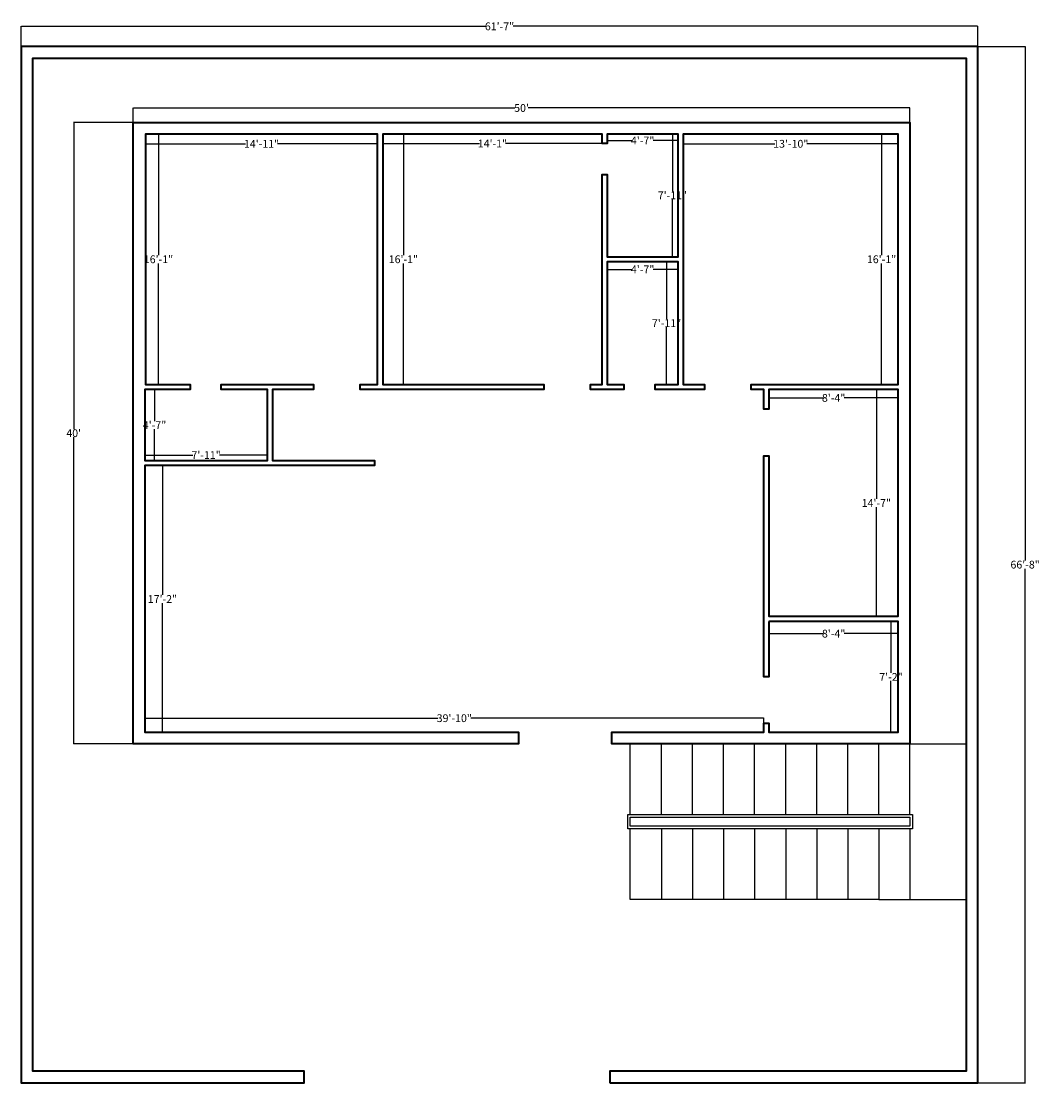
# Model space of a CAD drawing. Units: feet. Extents: x 3511 to 6270, y 2172 to 4127.
# Tile 1 of 4: x 3511 to 4297, y 3307 to 4127. Entities that reach past the tile are written whole.
import ezdxf

# ---------------------------------------------------------------- set-up
doc = ezdxf.new("R2010")
doc.units = ezdxf.units.FT
for name, color, linetype, lineweight in [('A-ANNO-DIMS', 2, 'Continuous', 18), ('A-FLOR-STRS', 4, 'Continuous', 25), ('A-WALL', 7, 'Continuous', 35), ('C-PROP', 1, 'Continuous', 35)]:
    doc.layers.add(name, color=color, linetype=linetype, lineweight=lineweight)
doc.styles.get("Standard").update_dxf_attribs({"font": 'arial.ttf'})
doc.dimstyles.get("Standard").update_dxf_attribs({"dimtxt": 6, "dimasz": 0.18, "dimexe": 0.18, "dimexo": 0.0625, "dimgap": 0.09, "dimtad": 0, "dimtih": 1, "dimtoh": 1, "dimdec": 0, "dimzin": 0, "dimdsep": 46, "dimlunit": 3, "dimtxsty": 'Standard', "dimcen": 0.09, "dimadec": 0, "dimazin": 0, "dimtfac": 1, "dimtdec": 0, "dimtofl": 0, "dimtmove": 0, "dimatfit": 3, "dimfxl": 1, "dimtolj": 1, "dimtzin": 0, "dimarcsym": 0})

# ---------------------------------------------------------------- blocks, each defined once
blk = doc.blocks.new('*D1')
at = {"layer": 'A-ANNO-DIMS', "color": 0, "lineweight": -2, "transparency": 16777216}
for p, q in [((3510.75, 4107.25), (3510.75, 4122.96)), ((3510.93, 4122.78), (3869.76, 4122.78)), ((4249.42, 4122.78), (3890.59, 4122.78)), ((4249.6, 4107.25), (4249.6, 4122.96))]:
    blk.add_line(p, q, dxfattribs=at)
at = {"layer": 'A-ANNO-DIMS', "color": 0, "transparency": 16777216}
for points in [[(3510.93, 4122.81), (3510.93, 4122.75), (3510.75, 4122.78)], [(4249.42, 4122.81), (4249.42, 4122.75), (4249.6, 4122.78)]]:
    blk.add_solid(points, dxfattribs=at)
at = {"layer": 'Defpoints', "color": 0, "transparency": 16777216}
for p in [(4249.6, 4122.78), (3510.75, 4107.19), (4249.6, 4107.19)]:
    blk.add_point(p, dxfattribs=at)
at = {"layer": 'A-ANNO-DIMS', "color": 0, "transparency": 16777216, "insert": (3880.17, 4122.78), "char_height": 6, "attachment_point": 5}
blk.add_mtext('\\A1;61\'-7"', dxfattribs=at)
blk = doc.blocks.new('*D2')
at = {"layer": 'A-ANNO-DIMS', "color": 0, "lineweight": -2, "transparency": 16777216}
for p, q in [((4249.67, 4107.19), (4286.32, 4107.19)), ((4286.14, 4107.01), (4286.14, 3710.22)), ((4286.14, 3307.12), (4286.14, 3703.91)), ((4249.67, 3306.94), (4286.32, 3306.94))]:
    blk.add_line(p, q, dxfattribs=at)
at = {"layer": 'A-ANNO-DIMS', "color": 0, "transparency": 16777216}
for points in [[(4286.11, 4107.01), (4286.17, 4107.01), (4286.14, 4107.19)], [(4286.11, 3307.12), (4286.17, 3307.12), (4286.14, 3306.94)]]:
    blk.add_solid(points, dxfattribs=at)
at = {"layer": 'Defpoints', "color": 0, "transparency": 16777216}
for p in [(4249.6, 4107.19), (4249.6, 3306.94), (4286.14, 3306.94)]:
    blk.add_point(p, dxfattribs=at)
at = {"layer": 'A-ANNO-DIMS', "color": 0, "transparency": 16777216, "insert": (4286.14, 3707.07), "char_height": 6, "attachment_point": 5}
blk.add_mtext('\\A1;66\'-8"', dxfattribs=at)
blk = doc.blocks.new('*D3')
at = {"layer": 'A-ANNO-DIMS', "color": 0, "lineweight": -2, "transparency": 16777216}
for p, q in [((3606.69, 4039.51), (3606.69, 4031.86)), ((3786.03, 4039.51), (3786.03, 4031.86)), ((3606.87, 4032.04), (3683.91, 4032.04)), ((3785.85, 4032.04), (3708.8, 4032.04))]:
    blk.add_line(p, q, dxfattribs=at)
at = {"layer": 'A-ANNO-DIMS', "color": 0, "transparency": 16777216}
for points in [[(3606.87, 4032.07), (3606.87, 4032.01), (3606.69, 4032.04)], [(3785.85, 4032.07), (3785.85, 4032.01), (3786.03, 4032.04)]]:
    blk.add_solid(points, dxfattribs=at)
at = {"layer": 'Defpoints', "color": 0, "transparency": 16777216}
for p in [(3606.69, 4039.58), (3786.03, 4039.58), (3786.03, 4032.04)]:
    blk.add_point(p, dxfattribs=at)
at = {"layer": 'A-ANNO-DIMS', "color": 0, "transparency": 16777216, "insert": (3696.36, 4032.04), "char_height": 6, "attachment_point": 5}
blk.add_mtext('\\A1;14\'-11"', dxfattribs=at)
blk = doc.blocks.new('*D4')
at = {"layer": 'A-ANNO-DIMS', "color": 0, "lineweight": -2, "transparency": 16777216}
for p, q in [((3606.75, 4039.58), (3616.96, 4039.58)), ((3616.78, 4039.4), (3616.78, 3946.05)), ((3616.78, 3846.39), (3616.78, 3939.74)), ((3606.75, 3846.21), (3616.96, 3846.21))]:
    blk.add_line(p, q, dxfattribs=at)
at = {"layer": 'A-ANNO-DIMS', "color": 0, "transparency": 16777216}
for points in [[(3616.75, 4039.4), (3616.81, 4039.4), (3616.78, 4039.58)], [(3616.75, 3846.39), (3616.81, 3846.39), (3616.78, 3846.21)]]:
    blk.add_solid(points, dxfattribs=at)
at = {"layer": 'Defpoints', "color": 0, "transparency": 16777216}
for p in [(3606.69, 4039.58), (3606.69, 3846.21), (3616.78, 3846.21)]:
    blk.add_point(p, dxfattribs=at)
at = {"layer": 'A-ANNO-DIMS', "color": 0, "transparency": 16777216, "insert": (3616.78, 3942.89), "char_height": 6, "attachment_point": 5}
blk.add_mtext('\\A1;16\'-1"', dxfattribs=at)
blk = doc.blocks.new('*D5')
at = {"layer": 'A-ANNO-DIMS', "color": 0, "lineweight": -2, "transparency": 16777216}
for p, q in [((3790.03, 4039.51), (3790.03, 4032.14)), ((3959.36, 4039.51), (3959.36, 4032.14)), ((3790.21, 4032.32), (3864.58, 4032.32)), ((3959.18, 4032.32), (3884.81, 4032.32))]:
    blk.add_line(p, q, dxfattribs=at)
at = {"layer": 'A-ANNO-DIMS', "color": 0, "transparency": 16777216}
for points in [[(3790.21, 4032.35), (3790.21, 4032.29), (3790.03, 4032.32)], [(3959.18, 4032.35), (3959.18, 4032.29), (3959.36, 4032.32)]]:
    blk.add_solid(points, dxfattribs=at)
at = {"layer": 'Defpoints', "color": 0, "transparency": 16777216}
for p in [(3790.03, 4039.58), (3959.36, 4039.58), (3959.36, 4032.32)]:
    blk.add_point(p, dxfattribs=at)
at = {"layer": 'A-ANNO-DIMS', "color": 0, "transparency": 16777216, "insert": (3874.7, 4032.32), "char_height": 6, "attachment_point": 5}
blk.add_mtext('\\A1;14\'-1"', dxfattribs=at)
blk = doc.blocks.new('*D6')
at = {"layer": 'A-ANNO-DIMS', "color": 0, "lineweight": -2, "transparency": 16777216}
for p, q in [((3790.09, 4039.58), (3806.12, 4039.58)), ((3805.94, 4039.4), (3805.94, 3946.05)), ((3805.94, 3846.39), (3805.94, 3939.74)), ((3790.09, 3846.21), (3806.12, 3846.21))]:
    blk.add_line(p, q, dxfattribs=at)
at = {"layer": 'A-ANNO-DIMS', "color": 0, "transparency": 16777216}
for points in [[(3805.91, 4039.4), (3805.97, 4039.4), (3805.94, 4039.58)], [(3805.91, 3846.39), (3805.97, 3846.39), (3805.94, 3846.21)]]:
    blk.add_solid(points, dxfattribs=at)
at = {"layer": 'Defpoints', "color": 0, "transparency": 16777216}
for p in [(3790.03, 4039.58), (3790.03, 3846.21), (3805.94, 3846.21)]:
    blk.add_point(p, dxfattribs=at)
at = {"layer": 'A-ANNO-DIMS', "color": 0, "transparency": 16777216, "insert": (3805.94, 3942.89), "char_height": 6, "attachment_point": 5}
blk.add_mtext('\\A1;16\'-1"', dxfattribs=at)
blk = doc.blocks.new('*D7')
at = {"layer": 'A-ANNO-DIMS', "color": 0, "lineweight": -2, "transparency": 16777216}
for p, q in [((3963.36, 4039.51), (3963.36, 4034.45)), ((3963.54, 4034.63), (3982.53, 4034.63)), ((4017.89, 4034.63), (3998.9, 4034.63)), ((4018.07, 4039.51), (4018.07, 4034.45))]:
    blk.add_line(p, q, dxfattribs=at)
at = {"layer": 'A-ANNO-DIMS', "color": 0, "transparency": 16777216}
for points in [[(3963.54, 4034.66), (3963.54, 4034.6), (3963.36, 4034.63)], [(4017.89, 4034.66), (4017.89, 4034.6), (4018.07, 4034.63)]]:
    blk.add_solid(points, dxfattribs=at)
at = {"layer": 'Defpoints', "color": 0, "transparency": 16777216}
for p in [(3963.36, 4039.58), (4018.07, 4039.58), (4018.07, 4034.63)]:
    blk.add_point(p, dxfattribs=at)
at = {"layer": 'A-ANNO-DIMS', "color": 0, "transparency": 16777216, "insert": (3990.72, 4034.63), "char_height": 6, "attachment_point": 5}
blk.add_mtext('\\A1;4\'-7"', dxfattribs=at)
blk = doc.blocks.new('*D8')
at = {"layer": 'A-ANNO-DIMS', "color": 0, "lineweight": -2, "transparency": 16777216}
for p, q in [((4018.01, 4039.58), (4013.55, 4039.58)), ((4013.73, 4039.4), (4013.73, 3995.34)), ((4013.73, 3945.07), (4013.73, 3989.13)), ((4018.01, 3944.89), (4013.55, 3944.89))]:
    blk.add_line(p, q, dxfattribs=at)
at = {"layer": 'A-ANNO-DIMS', "color": 0, "transparency": 16777216}
for points in [[(4013.7, 4039.4), (4013.76, 4039.4), (4013.73, 4039.58)], [(4013.7, 3945.07), (4013.76, 3945.07), (4013.73, 3944.89)]]:
    blk.add_solid(points, dxfattribs=at)
at = {"layer": 'Defpoints', "color": 0, "transparency": 16777216}
for p in [(4018.07, 4039.58), (4013.73, 3944.89), (4018.07, 3944.89)]:
    blk.add_point(p, dxfattribs=at)
at = {"layer": 'A-ANNO-DIMS', "color": 0, "transparency": 16777216, "insert": (4013.73, 3992.23), "char_height": 6, "attachment_point": 5}
blk.add_mtext('\\A1;7\'-11"', dxfattribs=at)
blk = doc.blocks.new('*D9')
at = {"layer": 'A-ANNO-DIMS', "color": 0, "lineweight": -2, "transparency": 16777216}
for p, q in [((4022.07, 4039.51), (4022.07, 4031.89)), ((4188.2, 4039.51), (4188.2, 4031.89)), ((4022.25, 4032.07), (4092.69, 4032.07)), ((4188.02, 4032.07), (4117.58, 4032.07))]:
    blk.add_line(p, q, dxfattribs=at)
at = {"layer": 'A-ANNO-DIMS', "color": 0, "transparency": 16777216}
for points in [[(4022.25, 4032.1), (4022.25, 4032.04), (4022.07, 4032.07)], [(4188.02, 4032.1), (4188.02, 4032.04), (4188.2, 4032.07)]]:
    blk.add_solid(points, dxfattribs=at)
at = {"layer": 'Defpoints', "color": 0, "transparency": 16777216}
for p in [(4022.07, 4039.58), (4188.2, 4039.58), (4188.2, 4032.07)]:
    blk.add_point(p, dxfattribs=at)
at = {"layer": 'A-ANNO-DIMS', "color": 0, "transparency": 16777216, "insert": (4105.13, 4032.07), "char_height": 6, "attachment_point": 5}
blk.add_mtext('\\A1;13\'-10"', dxfattribs=at)
blk = doc.blocks.new('*D10')
at = {"layer": 'A-ANNO-DIMS', "color": 0, "lineweight": -2, "transparency": 16777216}
for p, q in [((4188.14, 4039.58), (4175.08, 4039.58)), ((4175.26, 4039.4), (4175.26, 3946.05)), ((4175.26, 3846.39), (4175.26, 3939.74)), ((4188.14, 3846.21), (4175.08, 3846.21))]:
    blk.add_line(p, q, dxfattribs=at)
at = {"layer": 'A-ANNO-DIMS', "color": 0, "transparency": 16777216}
for points in [[(4175.23, 4039.4), (4175.29, 4039.4), (4175.26, 4039.58)], [(4175.23, 3846.39), (4175.29, 3846.39), (4175.26, 3846.21)]]:
    blk.add_solid(points, dxfattribs=at)
at = {"layer": 'Defpoints', "color": 0, "transparency": 16777216}
for p in [(4188.2, 4039.58), (4175.26, 3846.21), (4188.2, 3846.21)]:
    blk.add_point(p, dxfattribs=at)
at = {"layer": 'A-ANNO-DIMS', "color": 0, "transparency": 16777216, "insert": (4175.26, 3942.89), "char_height": 6, "attachment_point": 5}
blk.add_mtext('\\A1;16\'-1"', dxfattribs=at)
blk = doc.blocks.new('*D11')
at = {"layer": 'A-ANNO-DIMS', "color": 0, "lineweight": -2, "transparency": 16777216}
for p, q in [((4018.01, 3940.89), (4009, 3940.89)), ((4009.18, 3940.71), (4009.18, 3896.65)), ((4009.18, 3846.39), (4009.18, 3890.45)), ((4018.01, 3846.21), (4009, 3846.21))]:
    blk.add_line(p, q, dxfattribs=at)
at = {"layer": 'A-ANNO-DIMS', "color": 0, "transparency": 16777216}
for points in [[(4009.15, 3940.71), (4009.21, 3940.71), (4009.18, 3940.89)], [(4009.15, 3846.39), (4009.21, 3846.39), (4009.18, 3846.21)]]:
    blk.add_solid(points, dxfattribs=at)
at = {"layer": 'Defpoints', "color": 0, "transparency": 16777216}
for p in [(4018.07, 3940.89), (4009.18, 3846.21), (4018.07, 3846.21)]:
    blk.add_point(p, dxfattribs=at)
at = {"layer": 'A-ANNO-DIMS', "color": 0, "transparency": 16777216, "insert": (4009.18, 3893.55), "char_height": 6, "attachment_point": 5}
blk.add_mtext('\\A1;7\'-11"', dxfattribs=at)
blk = doc.blocks.new('*D12')
at = {"layer": 'A-ANNO-DIMS', "color": 0, "lineweight": -2, "transparency": 16777216}
for p, q in [((3963.36, 3940.83), (3963.36, 3934.92)), ((3963.54, 3935.1), (3982.53, 3935.1)), ((4017.89, 3935.1), (3998.9, 3935.1)), ((4018.07, 3940.83), (4018.07, 3934.92))]:
    blk.add_line(p, q, dxfattribs=at)
at = {"layer": 'A-ANNO-DIMS', "color": 0, "transparency": 16777216}
for points in [[(3963.54, 3935.13), (3963.54, 3935.07), (3963.36, 3935.1)], [(4017.89, 3935.13), (4017.89, 3935.07), (4018.07, 3935.1)]]:
    blk.add_solid(points, dxfattribs=at)
at = {"layer": 'Defpoints', "color": 0, "transparency": 16777216}
for p in [(3963.36, 3940.89), (4018.07, 3940.89), (4018.07, 3935.1)]:
    blk.add_point(p, dxfattribs=at)
at = {"layer": 'A-ANNO-DIMS', "color": 0, "transparency": 16777216, "insert": (3990.72, 3935.1), "char_height": 6, "attachment_point": 5}
blk.add_mtext('\\A1;4\'-7"', dxfattribs=at)
blk = doc.blocks.new('*D13')
at = {"layer": 'A-ANNO-DIMS', "color": 0, "lineweight": -2, "transparency": 16777216}
for p, q in [((3606.2, 3787.57), (3606.2, 3791.87)), ((3606.38, 3791.69), (3643.17, 3791.69)), ((3700.7, 3791.69), (3663.91, 3791.69)), ((3700.88, 3787.57), (3700.88, 3791.87))]:
    blk.add_line(p, q, dxfattribs=at)
at = {"layer": 'A-ANNO-DIMS', "color": 0, "transparency": 16777216}
for points in [[(3606.38, 3791.72), (3606.38, 3791.66), (3606.2, 3791.69)], [(3700.7, 3791.72), (3700.7, 3791.66), (3700.88, 3791.69)]]:
    blk.add_solid(points, dxfattribs=at)
at = {"layer": 'Defpoints', "color": 0, "transparency": 16777216}
for p in [(3606.2, 3787.5), (3700.88, 3791.69), (3700.88, 3787.5)]:
    blk.add_point(p, dxfattribs=at)
at = {"layer": 'A-ANNO-DIMS', "color": 0, "transparency": 16777216, "insert": (3653.54, 3791.69), "char_height": 6, "attachment_point": 5}
blk.add_mtext('\\A1;7\'-11"', dxfattribs=at)
blk = doc.blocks.new('*D14')
at = {"layer": 'A-ANNO-DIMS', "color": 0, "lineweight": -2, "transparency": 16777216}
for p, q in [((3606.26, 3842.21), (3613.9, 3842.21)), ((3613.72, 3842.03), (3613.72, 3817.95)), ((3613.72, 3787.68), (3613.72, 3811.77)), ((3606.26, 3787.5), (3613.9, 3787.5))]:
    blk.add_line(p, q, dxfattribs=at)
at = {"layer": 'A-ANNO-DIMS', "color": 0, "transparency": 16777216}
for points in [[(3613.69, 3842.03), (3613.75, 3842.03), (3613.72, 3842.21)], [(3613.69, 3787.68), (3613.75, 3787.68), (3613.72, 3787.5)]]:
    blk.add_solid(points, dxfattribs=at)
at = {"layer": 'Defpoints', "color": 0, "transparency": 16777216}
for p in [(3606.2, 3842.21), (3613.72, 3842.21), (3606.2, 3787.5)]:
    blk.add_point(p, dxfattribs=at)
at = {"layer": 'A-ANNO-DIMS', "color": 0, "transparency": 16777216, "insert": (3613.72, 3814.86), "char_height": 6, "attachment_point": 5}
blk.add_mtext('\\A1;4\'-7"', dxfattribs=at)
blk = doc.blocks.new('*D15')
at = {"layer": 'A-ANNO-DIMS', "color": 0, "lineweight": -2, "transparency": 16777216}
for p, q in [((3606.2, 3577.64), (3606.2, 3588.67)), ((3606.38, 3588.49), (3832.52, 3588.49)), ((4084.11, 3588.49), (3857.97, 3588.49)), ((4084.29, 3577.64), (4084.29, 3588.67))]:
    blk.add_line(p, q, dxfattribs=at)
at = {"layer": 'A-ANNO-DIMS', "color": 0, "transparency": 16777216}
for points in [[(3606.38, 3588.52), (3606.38, 3588.46), (3606.2, 3588.49)], [(4084.11, 3588.52), (4084.11, 3588.46), (4084.29, 3588.49)]]:
    blk.add_solid(points, dxfattribs=at)
at = {"layer": 'Defpoints', "color": 0, "transparency": 16777216}
for p in [(4084.29, 3588.49), (3606.2, 3577.58), (4084.29, 3577.58)]:
    blk.add_point(p, dxfattribs=at)
at = {"layer": 'A-ANNO-DIMS', "color": 0, "transparency": 16777216, "insert": (3845.24, 3588.49), "char_height": 6, "attachment_point": 5}
blk.add_mtext('\\A1;39\'-10"', dxfattribs=at)
blk = doc.blocks.new('*D16')
at = {"layer": 'A-ANNO-DIMS', "color": 0, "lineweight": -2, "transparency": 16777216}
for p, q in [((3606.26, 3783.5), (3620.02, 3783.5)), ((3619.84, 3783.32), (3619.84, 3683.64)), ((3619.84, 3577.76), (3619.84, 3677.44)), ((3606.26, 3577.58), (3620.02, 3577.58))]:
    blk.add_line(p, q, dxfattribs=at)
at = {"layer": 'A-ANNO-DIMS', "color": 0, "transparency": 16777216}
for points in [[(3619.81, 3783.32), (3619.87, 3783.32), (3619.84, 3783.5)], [(3619.81, 3577.76), (3619.87, 3577.76), (3619.84, 3577.58)]]:
    blk.add_solid(points, dxfattribs=at)
at = {"layer": 'Defpoints', "color": 0, "transparency": 16777216}
for p in [(3606.2, 3783.5), (3606.2, 3577.58), (3619.84, 3577.58)]:
    blk.add_point(p, dxfattribs=at)
at = {"layer": 'A-ANNO-DIMS', "color": 0, "transparency": 16777216, "insert": (3619.84, 3680.54), "char_height": 6, "attachment_point": 5}
blk.add_mtext('\\A1;17\'-2"', dxfattribs=at)
blk = doc.blocks.new('*D17')
at = {"layer": 'A-ANNO-DIMS', "color": 0, "lineweight": -2, "transparency": 16777216}
for p, q in [((4188.14, 3842.21), (4171.05, 3842.21)), ((4171.23, 3842.03), (4171.23, 3757.78)), ((4171.23, 3667.33), (4171.23, 3751.57)), ((4188.14, 3667.15), (4171.05, 3667.15))]:
    blk.add_line(p, q, dxfattribs=at)
at = {"layer": 'A-ANNO-DIMS', "color": 0, "transparency": 16777216}
for points in [[(4171.2, 3842.03), (4171.26, 3842.03), (4171.23, 3842.21)], [(4171.2, 3667.33), (4171.26, 3667.33), (4171.23, 3667.15)]]:
    blk.add_solid(points, dxfattribs=at)
at = {"layer": 'Defpoints', "color": 0, "transparency": 16777216}
for p in [(4188.2, 3842.21), (4171.23, 3667.15), (4188.2, 3667.15)]:
    blk.add_point(p, dxfattribs=at)
at = {"layer": 'A-ANNO-DIMS', "color": 0, "transparency": 16777216, "insert": (4171.23, 3754.68), "char_height": 6, "attachment_point": 5}
blk.add_mtext('\\A1;14\'-7"', dxfattribs=at)
blk = doc.blocks.new('*D18')
at = {"layer": 'A-ANNO-DIMS', "color": 0, "lineweight": -2, "transparency": 16777216}
for p, q in [((4088.29, 3842.15), (4088.29, 3835.65)), ((4188.2, 3842.15), (4188.2, 3835.65)), ((4088.47, 3835.83), (4130.18, 3835.83)), ((4188.02, 3835.83), (4146.31, 3835.83))]:
    blk.add_line(p, q, dxfattribs=at)
at = {"layer": 'A-ANNO-DIMS', "color": 0, "transparency": 16777216}
for points in [[(4088.47, 3835.86), (4088.47, 3835.8), (4088.29, 3835.83)], [(4188.02, 3835.86), (4188.02, 3835.8), (4188.2, 3835.83)]]:
    blk.add_solid(points, dxfattribs=at)
at = {"layer": 'Defpoints', "color": 0, "transparency": 16777216}
for p in [(4088.29, 3842.21), (4188.2, 3842.21), (4088.29, 3835.83)]:
    blk.add_point(p, dxfattribs=at)
at = {"layer": 'A-ANNO-DIMS', "color": 0, "transparency": 16777216, "insert": (4138.24, 3835.83), "char_height": 6, "attachment_point": 5}
blk.add_mtext('\\A1;8\'-4"', dxfattribs=at)
blk = doc.blocks.new('*D19')
at = {"layer": 'A-ANNO-DIMS', "color": 0, "lineweight": -2, "transparency": 16777216}
for p, q in [((4188.14, 3663.15), (4182.36, 3663.15)), ((4182.54, 3662.97), (4182.54, 3623.46)), ((4182.54, 3577.76), (4182.54, 3617.26)), ((4188.14, 3577.58), (4182.36, 3577.58))]:
    blk.add_line(p, q, dxfattribs=at)
at = {"layer": 'A-ANNO-DIMS', "color": 0, "transparency": 16777216}
for points in [[(4182.51, 3662.97), (4182.57, 3662.97), (4182.54, 3663.15)], [(4182.51, 3577.76), (4182.57, 3577.76), (4182.54, 3577.58)]]:
    blk.add_solid(points, dxfattribs=at)
at = {"layer": 'Defpoints', "color": 0, "transparency": 16777216}
for p in [(4188.2, 3663.15), (4182.54, 3577.58), (4188.2, 3577.58)]:
    blk.add_point(p, dxfattribs=at)
at = {"layer": 'A-ANNO-DIMS', "color": 0, "transparency": 16777216, "insert": (4182.54, 3620.36), "char_height": 6, "attachment_point": 5}
blk.add_mtext('\\A1;7\'-2"', dxfattribs=at)
blk = doc.blocks.new('*D20')
at = {"layer": 'A-ANNO-DIMS', "color": 0, "lineweight": -2, "transparency": 16777216}
for p, q in [((4088.29, 3663.08), (4088.29, 3653.6)), ((4188.2, 3663.08), (4188.2, 3653.6)), ((4088.47, 3653.78), (4130.18, 3653.78)), ((4188.02, 3653.78), (4146.31, 3653.78))]:
    blk.add_line(p, q, dxfattribs=at)
at = {"layer": 'A-ANNO-DIMS', "color": 0, "transparency": 16777216}
for points in [[(4088.47, 3653.81), (4088.47, 3653.75), (4088.29, 3653.78)], [(4188.02, 3653.81), (4188.02, 3653.75), (4188.2, 3653.78)]]:
    blk.add_solid(points, dxfattribs=at)
at = {"layer": 'Defpoints', "color": 0, "transparency": 16777216}
for p in [(4088.29, 3663.15), (4188.2, 3663.15), (4088.29, 3653.78)]:
    blk.add_point(p, dxfattribs=at)
at = {"layer": 'A-ANNO-DIMS', "color": 0, "transparency": 16777216, "insert": (4138.24, 3653.78), "char_height": 6, "attachment_point": 5}
blk.add_mtext('\\A1;8\'-4"', dxfattribs=at)
blk = doc.blocks.new('*D21')
at = {"layer": 'A-ANNO-DIMS', "color": 0, "lineweight": -2, "transparency": 16777216}
for p, q in [((3597.14, 4048.58), (3551.09, 4048.58)), ((3551.27, 4048.4), (3551.27, 3811.73)), ((3551.27, 3568.76), (3551.27, 3805.42)), ((3597.14, 3568.58), (3551.09, 3568.58))]:
    blk.add_line(p, q, dxfattribs=at)
at = {"layer": 'A-ANNO-DIMS', "color": 0, "transparency": 16777216}
for points in [[(3551.24, 4048.4), (3551.3, 4048.4), (3551.27, 4048.58)], [(3551.24, 3568.76), (3551.3, 3568.76), (3551.27, 3568.58)]]:
    blk.add_solid(points, dxfattribs=at)
at = {"layer": 'Defpoints', "color": 0, "transparency": 16777216}
for p in [(3597.2, 4048.58), (3551.27, 3568.58), (3597.2, 3568.58)]:
    blk.add_point(p, dxfattribs=at)
at = {"layer": 'A-ANNO-DIMS', "color": 0, "transparency": 16777216, "insert": (3551.27, 3808.58), "char_height": 6, "attachment_point": 5}
blk.add_mtext("\\A1;40'", dxfattribs=at)
blk = doc.blocks.new('*D22')
at = {"layer": 'A-ANNO-DIMS', "color": 0, "lineweight": -2, "transparency": 16777216}
for p, q in [((3597.2, 4048.64), (3597.2, 4059.92)), ((3597.38, 4059.74), (3892.02, 4059.74)), ((4197.02, 4059.74), (3902.38, 4059.74)), ((4197.2, 4048.64), (4197.2, 4059.92))]:
    blk.add_line(p, q, dxfattribs=at)
at = {"layer": 'A-ANNO-DIMS', "color": 0, "transparency": 16777216}
for points in [[(3597.38, 4059.77), (3597.38, 4059.71), (3597.2, 4059.74)], [(4197.02, 4059.77), (4197.02, 4059.71), (4197.2, 4059.74)]]:
    blk.add_solid(points, dxfattribs=at)
at = {"layer": 'Defpoints', "color": 0, "transparency": 16777216}
for p in [(4197.2, 4059.74), (3597.2, 4048.58), (4197.2, 4048.58)]:
    blk.add_point(p, dxfattribs=at)
at = {"layer": 'A-ANNO-DIMS', "color": 0, "transparency": 16777216, "insert": (3897.2, 4059.74), "char_height": 6, "attachment_point": 5}
blk.add_mtext("\\A1;50'", dxfattribs=at)
blk = doc.blocks.new('STAIR')
for p, q in [((2, 65.57), (2, 120)), ((26, 65.57), (26, 120)), ((50, 65.57), (50, 120)), ((74, 65.57), (74, 120)), ((98, 65.57), (98, 120)), ((122, 65.57), (122, 120)), ((146, 65.57), (146, 120)), ((170, 65.57), (170, 120)), ((194, 65.57), (194, 120)), ((218, 54.42), (218, 0))]:
    blk.add_line(p, q)
for points in [[(218, 65.57), (218, 120), (261.4, 120)], [(26, 54.42), (26, 0), (14, 0), (2, 0), (2, 54.42)], [(50, 54.42), (50, 0), (38, 0), (26, 0)], [(74, 54.42), (74, 0), (62, 0), (50, 0)], [(98, 54.42), (98, 0), (86, 0), (74, 0)], [(122, 54.42), (122, 0), (110, 0), (98, 0)], [(146, 54.42), (146, 0), (134, 0), (122, 0)], [(170, 54.42), (170, 0), (158, 0), (146, 0)], [(194, 54.42), (194, 0), (182, 0), (170, 0)], [(194, 0), (206, 0), (218, 0), (261.4, 0)]]:
    blk.add_lwpolyline(points)
for points in [[(0, 65.57), (220, 65.57), (220, 54.42), (0, 54.42)], [(218, 56.42), (2, 56.42), (2, 63.57), (218, 63.57)]]:
    blk.add_lwpolyline(points, close=True)

msp = doc.modelspace()

# ---------------------------------------------------------------- linework, layer by layer
at = {"layer": 'A-WALL'}
msp.add_lwpolyline([(4088.29, 3663.15), (4088.29, 3620.52), (4084.29, 3620.52), (4084.29, 3791.14), (4088.29, 3791.14), (4088.29, 3667.15), (4188.2, 3667.15), (4188.2, 3842.21), (4088.29, 3842.21), (4088.29, 3827.14), (4084.29, 3827.14), (4084.29, 3842.21), (4074.6, 3842.21), (4074.6, 3846.21), (4188.2, 3846.21), (4188.2, 4039.58), (4022.07, 4039.58), (4022.07, 3846.21), (4038.6, 3846.21), (4038.6, 3842.21), (4000.3, 3842.21), (4000.3, 3846.21), (4018.07, 3846.21), (4018.07, 3940.89), (3963.36, 3940.89), (3963.36, 3846.21), (3976.3, 3846.21), (3976.3, 3842.21), (3950.36, 3842.21), (3950.36, 3846.21), (3959.36, 3846.21), (3959.36, 4008.32), (3963.36, 4008.32), (3963.36, 3944.89), (4018.07, 3944.89), (4018.07, 4039.58), (3963.36, 4039.58), (3963.36, 4032.32), (3959.36, 4032.32), (3959.36, 4039.58), (3790.03, 4039.58), (3790.03, 3846.21), (3914.36, 3846.21), (3914.36, 3842.21), (3772.46, 3842.21), (3772.46, 3846.21), (3786.03, 3846.21), (3786.03, 4039.58), (3606.69, 4039.58), (3606.69, 3846.21), (3641.22, 3846.21), (3641.22, 3842.21), (3606.2, 3842.21), (3606.2, 3787.5), (3606.2, 3787.5), (3700.88, 3787.5), (3700.88, 3842.21), (3665.22, 3842.21), (3665.22, 3846.21), (3736.46, 3846.21), (3736.46, 3842.21), (3704.88, 3842.21), (3704.88, 3787.51), (3783.64, 3787.51), (3783.64, 3783.5), (3606.2, 3783.5), (3606.2, 3577.58), (3894.84, 3577.58), (3894.84, 3568.58), (3597.2, 3568.58), (3597.2, 4048.58), (4197.2, 4048.58), (4197.2, 3568.58), (3966.84, 3568.58), (3966.84, 3577.58), (4084.29, 3577.58), (4084.29, 3584.52), (4088.29, 3584.52), (4088.29, 3577.58), (4188.2, 3577.58), (4188.2, 3663.15)], close=True, dxfattribs=at)
msp.add_lwpolyline([(3704.88, 3783.5), (3704.88, 3783.5)], dxfattribs=at)
at = {"layer": 'C-PROP'}
msp.add_lwpolyline([(3965.44, 3306.94), (4249.6, 3306.94), (4249.6, 4107.19), (3510.75, 4107.19), (3510.75, 3306.94), (3729.37, 3306.94), (3729.37, 3315.94), (3519.75, 3315.94), (3519.75, 4098.19), (4240.6, 4098.19), (4240.6, 3315.94), (3965.44, 3315.94)], close=True, dxfattribs=at)

# ---------------------------------------------------------------- block references
at = {"layer": 'A-FLOR-STRS'}
msp.add_blockref('STAIR', (3979.2, 3448.58), dxfattribs=at)

# ---------------------------------------------------------------- dimensions: what is measured, and where the dimension line sits
at = {"layer": 'A-ANNO-DIMS'}
for base, p1, p2, picture, middle in [((4249.6, 4122.78), (3510.75, 4107.19), (4249.6, 4107.19), '*D1', (3880.17, 4122.78)), ((4197.2, 4059.74), (3597.2, 4048.58), (4197.2, 4048.58), '*D22', (3897.2, 4059.74)), ((3786.03, 4032.04), (3606.69, 4039.58), (3786.03, 4039.58), '*D3', (3696.36, 4032.04)), ((3959.36, 4032.32), (3790.03, 4039.58), (3959.36, 4039.58), '*D5', (3874.7, 4032.32)), ((4018.07, 4034.63), (3963.36, 4039.58), (4018.07, 4039.58), '*D7', (3990.72, 4034.63)), ((4188.2, 4032.07), (4022.07, 4039.58), (4188.2, 4039.58), '*D9', (4105.13, 4032.07)), ((4018.07, 3935.1), (3963.36, 3940.89), (4018.07, 3940.89), '*D12', (3990.72, 3935.1)), ((4088.29, 3835.83), (4188.2, 3842.21), (4088.29, 3842.21), '*D18', (4138.24, 3835.83)), ((3700.88, 3791.69), (3606.2, 3787.5), (3700.88, 3787.5), '*D13', (3653.54, 3791.69)), ((4088.29, 3653.78), (4188.2, 3663.15), (4088.29, 3663.15), '*D20', (4138.24, 3653.78)), ((4084.29, 3588.49), (3606.2, 3577.58), (4084.29, 3577.58), '*D15', (3845.24, 3588.49))]:
    dim = msp.add_linear_dim(base=base, p1=p1, p2=p2, dimstyle='Standard', override={"dimclrd": 0, "dimclre": 0, "dimclrt": 0}, dxfattribs=at)
    dim.commit()
    dim.dimension.update_dxf_attribs({"geometry": picture, "text_midpoint": middle})
for base, p1, p2, picture, middle in [((4286.14, 3306.94), (4249.6, 4107.19), (4249.6, 3306.94), '*D2', (4286.14, 3707.07)), ((3551.27, 3568.58), (3597.2, 4048.58), (3597.2, 3568.58), '*D21', (3551.27, 3808.58)), ((3616.78, 3846.21), (3606.69, 4039.58), (3606.69, 3846.21), '*D4', (3616.78, 3942.89)), ((3805.94, 3846.21), (3790.03, 4039.58), (3790.03, 3846.21), '*D6', (3805.94, 3942.89)), ((4013.73, 3944.89), (4018.07, 4039.58), (4018.07, 3944.89), '*D8', (4013.73, 3992.23)), ((4175.26, 3846.21), (4188.2, 4039.58), (4188.2, 3846.21), '*D10', (4175.26, 3942.89)), ((4009.18, 3846.21), (4018.07, 3940.89), (4018.07, 3846.21), '*D11', (4009.18, 3893.55)), ((3613.72, 3842.21), (3606.2, 3787.5), (3606.2, 3842.21), '*D14', (3613.72, 3814.86)), ((4171.23, 3667.15), (4188.2, 3842.21), (4188.2, 3667.15), '*D17', (4171.23, 3754.68)), ((3619.84, 3577.58), (3606.2, 3783.5), (3606.2, 3577.58), '*D16', (3619.84, 3680.54)), ((4182.54, 3577.58), (4188.2, 3663.15), (4188.2, 3577.58), '*D19', (4182.54, 3620.36))]:
    dim = msp.add_linear_dim(base=base, p1=p1, p2=p2, angle=90, dimstyle='Standard', override={"dimclrd": 0, "dimclre": 0, "dimclrt": 0}, dxfattribs=at)
    dim.commit()
    dim.dimension.update_dxf_attribs({"geometry": picture, "text_midpoint": middle})

doc.saveas('drawing.dxf')
